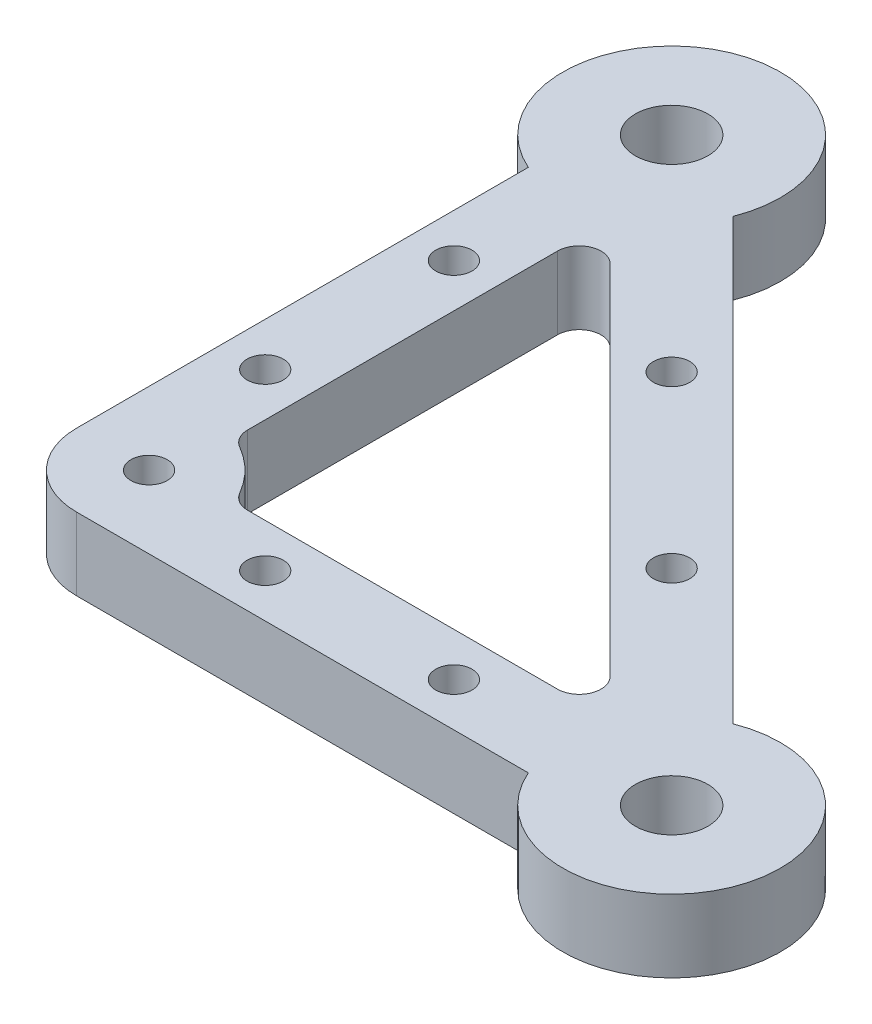
ISO-10303-21;
HEADER;
FILE_DESCRIPTION(('STEP AP214'),'2;1');
FILE_NAME('part.step','',(''),(''),'','','');
FILE_SCHEMA(('AUTOMOTIVE_DESIGN { 1 0 10303 214 1 1 1 1 }'));
ENDSEC;
DATA;
#1=APPLICATION_CONTEXT('core data for automotive mechanical design processes');
#2=APPLICATION_PROTOCOL_DEFINITION('international standard','automotive_design',2000,#1);
#3=PRODUCT_CONTEXT('',#1,'mechanical');
#4=PRODUCT('Part','Part','',(#3));
#5=PRODUCT_RELATED_PRODUCT_CATEGORY('part','',(#4));
#6=PRODUCT_DEFINITION_FORMATION('','',#4);
#7=PRODUCT_DEFINITION_CONTEXT('part definition',#1,'design');
#8=PRODUCT_DEFINITION('design','',#6,#7);
#9=PRODUCT_DEFINITION_SHAPE('','',#8);
#10=(LENGTH_UNIT() NAMED_UNIT(*) SI_UNIT(.MILLI.,.METRE.));
#11=(NAMED_UNIT(*) PLANE_ANGLE_UNIT() SI_UNIT($,.RADIAN.));
#12=(NAMED_UNIT(*) SI_UNIT($,.STERADIAN.) SOLID_ANGLE_UNIT());
#13=UNCERTAINTY_MEASURE_WITH_UNIT(LENGTH_MEASURE(1.E-05),#10,'distance_accuracy_value','');
#14=(GEOMETRIC_REPRESENTATION_CONTEXT(3) GLOBAL_UNCERTAINTY_ASSIGNED_CONTEXT((#13)) GLOBAL_UNIT_ASSIGNED_CONTEXT((#10,
#11,#12)) REPRESENTATION_CONTEXT('',''));
#15=CARTESIAN_POINT('',(0.,0.,0.));
#16=DIRECTION('',(0.,0.,1.));
#17=DIRECTION('',(1.,0.,0.));
#18=AXIS2_PLACEMENT_3D('',#15,#16,#17);
#19=CARTESIAN_POINT('',(4.,5.,-4.));
#20=DIRECTION('',(0.,1.,0.));
#21=DIRECTION('',(0.,0.,1.));
#22=AXIS2_PLACEMENT_3D('',#19,#20,#21);
#23=PLANE('',#22);
#24=CARTESIAN_POINT('',(28.2842712474619,5.,-51.7157287525381));
#25=DIRECTION('',(0.,1.,0.));
#26=DIRECTION('',(0.,0.,1.));
#27=AXIS2_PLACEMENT_3D('',#24,#25,#26);
#28=CIRCLE('',#27,2.5);
#29=CARTESIAN_POINT('',(28.2842712474619,5.,-49.2157287525381));
#30=VERTEX_POINT('',#29);
#31=EDGE_CURVE('E389',#30,#30,#28,.T.);
#32=ORIENTED_EDGE('',*,*,#31,.F.);
#33=EDGE_LOOP('',(#32));
#34=FACE_BOUND('',#33,.T.);
#35=CARTESIAN_POINT('',(0.,5.,-24.));
#36=DIRECTION('',(0.,1.,0.));
#37=DIRECTION('',(0.,0.,1.));
#38=AXIS2_PLACEMENT_3D('',#35,#36,#37);
#39=CIRCLE('',#38,2.5);
#40=CARTESIAN_POINT('',(0.,5.,-21.5));
#41=VERTEX_POINT('',#40);
#42=EDGE_CURVE('E398',#41,#41,#39,.T.);
#43=ORIENTED_EDGE('',*,*,#42,.F.);
#44=EDGE_LOOP('',(#43));
#45=FACE_BOUND('',#44,.T.);
#46=CARTESIAN_POINT('',(50.,5.,0.));
#47=DIRECTION('',(0.,1.,0.));
#48=DIRECTION('',(0.,0.,1.));
#49=AXIS2_PLACEMENT_3D('',#46,#47,#48);
#50=CIRCLE('',#49,2.5);
#51=CARTESIAN_POINT('',(50.,5.,2.5));
#52=VERTEX_POINT('',#51);
#53=EDGE_CURVE('E179',#52,#52,#50,.T.);
#54=ORIENTED_EDGE('',*,*,#53,.F.);
#55=EDGE_LOOP('',(#54));
#56=FACE_BOUND('',#55,.T.);
#57=CARTESIAN_POINT('',(0.,5.,-80.));
#58=DIRECTION('',(0.,1.,0.));
#59=DIRECTION('',(0.,0.,1.));
#60=AXIS2_PLACEMENT_3D('',#57,#58,#59);
#61=CIRCLE('',#60,5.);
#62=CARTESIAN_POINT('',(0.,5.,-75.));
#63=VERTEX_POINT('',#62);
#64=EDGE_CURVE('E212',#63,#63,#61,.T.);
#65=ORIENTED_EDGE('',*,*,#64,.F.);
#66=EDGE_LOOP('',(#65));
#67=FACE_BOUND('',#66,.T.);
#68=CARTESIAN_POINT('',(4.,5.,-4.));
#69=DIRECTION('',(0.,1.,0.));
#70=DIRECTION('',(0.,0.,1.));
#71=AXIS2_PLACEMENT_3D('',#68,#69,#70);
#72=CIRCLE('',#71,10.);
#73=CARTESIAN_POINT('',(-6.,5.,-4.));
#74=VERTEX_POINT('',#73);
#75=CARTESIAN_POINT('',(4.,5.,6.));
#76=VERTEX_POINT('',#75);
#77=EDGE_CURVE('E227',#74,#76,#72,.T.);
#78=ORIENTED_EDGE('',*,*,#77,.T.);
#79=DIRECTION('',(1.,0.,0.));
#80=VECTOR('',#79,1.);
#81=CARTESIAN_POINT('',(4.,5.,6.));
#82=LINE('',#81,#80);
#83=CARTESIAN_POINT('',(66.2522729151325,5.,5.99999999999999));
#84=VERTEX_POINT('',#83);
#85=EDGE_CURVE('E226',#76,#84,#82,.T.);
#86=ORIENTED_EDGE('',*,*,#85,.T.);
#87=CARTESIAN_POINT('',(80.,5.,0.));
#88=DIRECTION('',(0.,1.,0.));
#89=DIRECTION('',(0.,0.,1.));
#90=AXIS2_PLACEMENT_3D('',#87,#88,#89);
#91=CIRCLE('',#90,15.);
#92=CARTESIAN_POINT('',(74.5215296395075,5.,-13.9637517347311));
#93=VERTEX_POINT('',#92);
#94=EDGE_CURVE('E235',#84,#93,#91,.T.);
#95=ORIENTED_EDGE('',*,*,#94,.T.);
#96=DIRECTION('',(-0.707106781186547,0.,-0.707106781186547));
#97=VECTOR('',#96,1.);
#98=CARTESIAN_POINT('',(13.9637517347311,5.,-74.5215296395075));
#99=LINE('',#98,#97);
#100=CARTESIAN_POINT('',(13.9637517347311,5.,-74.5215296395075));
#101=VERTEX_POINT('',#100);
#102=EDGE_CURVE('E231',#93,#101,#99,.T.);
#103=ORIENTED_EDGE('',*,*,#102,.T.);
#104=CARTESIAN_POINT('',(0.,5.,-80.));
#105=DIRECTION('',(0.,1.,0.));
#106=DIRECTION('',(0.,0.,1.));
#107=AXIS2_PLACEMENT_3D('',#104,#105,#106);
#108=CIRCLE('',#107,15.);
#109=CARTESIAN_POINT('',(-6.,5.,-66.2522729151325));
#110=VERTEX_POINT('',#109);
#111=EDGE_CURVE('E237',#101,#110,#108,.T.);
#112=ORIENTED_EDGE('',*,*,#111,.T.);
#113=DIRECTION('',(0.,0.,1.));
#114=VECTOR('',#113,1.);
#115=CARTESIAN_POINT('',(-6.,5.,-4.));
#116=LINE('',#115,#114);
#117=EDGE_CURVE('E236',#110,#74,#116,.T.);
#118=ORIENTED_EDGE('',*,*,#117,.T.);
#119=EDGE_LOOP('',(#78,#86,#95,#103,#112,#118));
#120=FACE_BOUND('',#119,.T.);
#121=CARTESIAN_POINT('',(80.,5.,0.));
#122=DIRECTION('',(0.,1.,0.));
#123=DIRECTION('',(0.,0.,1.));
#124=AXIS2_PLACEMENT_3D('',#121,#122,#123);
#125=CIRCLE('',#124,5.);
#126=CARTESIAN_POINT('',(80.,5.,5.));
#127=VERTEX_POINT('',#126);
#128=EDGE_CURVE('E219',#127,#127,#125,.T.);
#129=ORIENTED_EDGE('',*,*,#128,.F.);
#130=EDGE_LOOP('',(#129));
#131=FACE_BOUND('',#130,.T.);
#132=CARTESIAN_POINT('',(4.,5.,-4.));
#133=DIRECTION('',(0.,1.,0.));
#134=DIRECTION('',(0.,0.,1.));
#135=AXIS2_PLACEMENT_3D('',#132,#133,#134);
#136=CIRCLE('',#135,2.5);
#137=CARTESIAN_POINT('',(4.,5.,-1.5));
#138=VERTEX_POINT('',#137);
#139=EDGE_CURVE('E208',#138,#138,#136,.T.);
#140=ORIENTED_EDGE('',*,*,#139,.F.);
#141=EDGE_LOOP('',(#140));
#142=FACE_BOUND('',#141,.T.);
#143=DIRECTION('',(1.,0.,0.));
#144=VECTOR('',#143,1.);
#145=CARTESIAN_POINT('',(15.5884572681199,5.,-6.));
#146=LINE('',#145,#144);
#147=CARTESIAN_POINT('',(15.5884572681199,5.,-6.));
#148=VERTEX_POINT('',#147);
#149=CARTESIAN_POINT('',(58.2720779386422,5.,-6.));
#150=VERTEX_POINT('',#149);
#151=EDGE_CURVE('E146',#148,#150,#146,.T.);
#152=ORIENTED_EDGE('',*,*,#151,.F.);
#153=CARTESIAN_POINT('',(15.5884572681199,5.,-9.));
#154=DIRECTION('',(0.,1.,0.));
#155=DIRECTION('',(0.,0.,-1.));
#156=AXIS2_PLACEMENT_3D('',#153,#154,#155);
#157=CIRCLE('',#156,3.);
#158=CARTESIAN_POINT('',(12.9903810567666,5.,-7.5));
#159=VERTEX_POINT('',#158);
#160=EDGE_CURVE('E138',#159,#148,#157,.T.);
#161=ORIENTED_EDGE('',*,*,#160,.F.);
#162=CARTESIAN_POINT('',(0.,5.,0.));
#163=DIRECTION('',(0.,-1.,0.));
#164=DIRECTION('',(0.,0.,1.));
#165=AXIS2_PLACEMENT_3D('',#162,#163,#164);
#166=CIRCLE('',#165,15.);
#167=CARTESIAN_POINT('',(7.5,5.,-12.9903810567666));
#168=VERTEX_POINT('',#167);
#169=EDGE_CURVE('E173',#168,#159,#166,.T.);
#170=ORIENTED_EDGE('',*,*,#169,.F.);
#171=CARTESIAN_POINT('',(9.,5.,-15.5884572681199));
#172=DIRECTION('',(0.,1.,0.));
#173=DIRECTION('',(0.,0.,-1.));
#174=AXIS2_PLACEMENT_3D('',#171,#172,#173);
#175=CIRCLE('',#174,3.);
#176=CARTESIAN_POINT('',(6.,5.,-15.5884572681199));
#177=VERTEX_POINT('',#176);
#178=EDGE_CURVE('E174',#177,#168,#175,.T.);
#179=ORIENTED_EDGE('',*,*,#178,.F.);
#180=DIRECTION('',(0.,0.,1.));
#181=VECTOR('',#180,1.);
#182=CARTESIAN_POINT('',(6.,5.,-15.5884572681199));
#183=LINE('',#182,#181);
#184=CARTESIAN_POINT('',(6.,5.,-58.2720779386421));
#185=VERTEX_POINT('',#184);
#186=EDGE_CURVE('E172',#185,#177,#183,.T.);
#187=ORIENTED_EDGE('',*,*,#186,.F.);
#188=CARTESIAN_POINT('',(9.,5.,-58.2720779386421));
#189=DIRECTION('',(0.,1.,0.));
#190=DIRECTION('',(0.,0.,1.));
#191=AXIS2_PLACEMENT_3D('',#188,#189,#190);
#192=CIRCLE('',#191,3.);
#193=CARTESIAN_POINT('',(11.1213203435596,5.,-60.3933982822018));
#194=VERTEX_POINT('',#193);
#195=EDGE_CURVE('E166',#194,#185,#192,.T.);
#196=ORIENTED_EDGE('',*,*,#195,.F.);
#197=DIRECTION('',(-0.707106781186547,0.,-0.707106781186547));
#198=VECTOR('',#197,1.);
#199=CARTESIAN_POINT('',(11.1213203435596,5.,-60.3933982822018));
#200=LINE('',#199,#198);
#201=CARTESIAN_POINT('',(60.3933982822018,5.,-11.1213203435596));
#202=VERTEX_POINT('',#201);
#203=EDGE_CURVE('E163',#202,#194,#200,.T.);
#204=ORIENTED_EDGE('',*,*,#203,.F.);
#205=CARTESIAN_POINT('',(58.2720779386422,5.,-9.));
#206=DIRECTION('',(0.,1.,0.));
#207=DIRECTION('',(0.,0.,1.));
#208=AXIS2_PLACEMENT_3D('',#205,#206,#207);
#209=CIRCLE('',#208,3.);
#210=EDGE_CURVE('E165',#150,#202,#209,.T.);
#211=ORIENTED_EDGE('',*,*,#210,.F.);
#212=EDGE_LOOP('',(#152,#161,#170,#179,#187,#196,#204,#211));
#213=FACE_BOUND('',#212,.T.);
#214=CARTESIAN_POINT('',(24.,5.,0.));
#215=DIRECTION('',(0.,1.,0.));
#216=DIRECTION('',(0.,0.,1.));
#217=AXIS2_PLACEMENT_3D('',#214,#215,#216);
#218=CIRCLE('',#217,2.5);
#219=CARTESIAN_POINT('',(24.,5.,2.5));
#220=VERTEX_POINT('',#219);
#221=EDGE_CURVE('E407',#220,#220,#218,.T.);
#222=ORIENTED_EDGE('',*,*,#221,.F.);
#223=EDGE_LOOP('',(#222));
#224=FACE_BOUND('',#223,.T.);
#225=CARTESIAN_POINT('',(0.,5.,-50.));
#226=DIRECTION('',(0.,1.,0.));
#227=DIRECTION('',(0.,0.,1.));
#228=AXIS2_PLACEMENT_3D('',#225,#226,#227);
#229=CIRCLE('',#228,2.5);
#230=CARTESIAN_POINT('',(0.,5.,-47.5));
#231=VERTEX_POINT('',#230);
#232=EDGE_CURVE('E391',#231,#231,#229,.T.);
#233=ORIENTED_EDGE('',*,*,#232,.F.);
#234=EDGE_LOOP('',(#233));
#235=FACE_BOUND('',#234,.T.);
#236=CARTESIAN_POINT('',(51.7157287525381,5.,-28.2842712474619));
#237=DIRECTION('',(0.,1.,0.));
#238=DIRECTION('',(0.,0.,1.));
#239=AXIS2_PLACEMENT_3D('',#236,#237,#238);
#240=CIRCLE('',#239,2.5);
#241=CARTESIAN_POINT('',(51.7157287525381,5.,-25.7842712474619));
#242=VERTEX_POINT('',#241);
#243=EDGE_CURVE('E377',#242,#242,#240,.T.);
#244=ORIENTED_EDGE('',*,*,#243,.F.);
#245=EDGE_LOOP('',(#244));
#246=FACE_BOUND('',#245,.T.);
#247=ADVANCED_FACE('F39',(#34,#45,#56,#67,#120,#131,#142,#213,#224,#235,#246),#23,.T.);
#248=CARTESIAN_POINT('',(4.,-5.,-4.));
#249=DIRECTION('',(0.,1.,0.));
#250=DIRECTION('',(0.,0.,1.));
#251=AXIS2_PLACEMENT_3D('',#248,#249,#250);
#252=PLANE('',#251);
#253=CARTESIAN_POINT('',(4.,-5.,-4.));
#254=DIRECTION('',(0.,1.,0.));
#255=DIRECTION('',(0.,0.,1.));
#256=AXIS2_PLACEMENT_3D('',#253,#254,#255);
#257=CIRCLE('',#256,2.5);
#258=CARTESIAN_POINT('',(4.,-5.,-1.5));
#259=VERTEX_POINT('',#258);
#260=EDGE_CURVE('E156',#259,#259,#257,.T.);
#261=ORIENTED_EDGE('',*,*,#260,.T.);
#262=EDGE_LOOP('',(#261));
#263=FACE_BOUND('',#262,.T.);
#264=CARTESIAN_POINT('',(0.,-5.,-80.));
#265=DIRECTION('',(0.,1.,0.));
#266=DIRECTION('',(0.,0.,1.));
#267=AXIS2_PLACEMENT_3D('',#264,#265,#266);
#268=CIRCLE('',#267,5.);
#269=CARTESIAN_POINT('',(0.,-5.,-75.));
#270=VERTEX_POINT('',#269);
#271=EDGE_CURVE('E211',#270,#270,#268,.T.);
#272=ORIENTED_EDGE('',*,*,#271,.T.);
#273=EDGE_LOOP('',(#272));
#274=FACE_BOUND('',#273,.T.);
#275=CARTESIAN_POINT('',(80.,-5.,0.));
#276=DIRECTION('',(0.,1.,0.));
#277=DIRECTION('',(0.,0.,1.));
#278=AXIS2_PLACEMENT_3D('',#275,#276,#277);
#279=CIRCLE('',#278,5.);
#280=CARTESIAN_POINT('',(80.,-5.,5.));
#281=VERTEX_POINT('',#280);
#282=EDGE_CURVE('E220',#281,#281,#279,.T.);
#283=ORIENTED_EDGE('',*,*,#282,.T.);
#284=EDGE_LOOP('',(#283));
#285=FACE_BOUND('',#284,.T.);
#286=CARTESIAN_POINT('',(4.,-5.,-4.));
#287=DIRECTION('',(0.,1.,0.));
#288=DIRECTION('',(0.,0.,1.));
#289=AXIS2_PLACEMENT_3D('',#286,#287,#288);
#290=CIRCLE('',#289,10.);
#291=CARTESIAN_POINT('',(-6.,-5.,-4.));
#292=VERTEX_POINT('',#291);
#293=CARTESIAN_POINT('',(4.,-5.,6.));
#294=VERTEX_POINT('',#293);
#295=EDGE_CURVE('E224',#292,#294,#290,.T.);
#296=ORIENTED_EDGE('',*,*,#295,.F.);
#297=DIRECTION('',(0.,0.,1.));
#298=VECTOR('',#297,1.);
#299=CARTESIAN_POINT('',(-6.,-5.,-4.));
#300=LINE('',#299,#298);
#301=CARTESIAN_POINT('',(-6.,-5.,-66.2522729151325));
#302=VERTEX_POINT('',#301);
#303=EDGE_CURVE('E228',#302,#292,#300,.T.);
#304=ORIENTED_EDGE('',*,*,#303,.F.);
#305=CARTESIAN_POINT('',(0.,-5.,-80.));
#306=DIRECTION('',(0.,1.,0.));
#307=DIRECTION('',(0.,0.,1.));
#308=AXIS2_PLACEMENT_3D('',#305,#306,#307);
#309=CIRCLE('',#308,15.);
#310=CARTESIAN_POINT('',(13.9637517347311,-5.,-74.5215296395075));
#311=VERTEX_POINT('',#310);
#312=EDGE_CURVE('E246',#311,#302,#309,.T.);
#313=ORIENTED_EDGE('',*,*,#312,.F.);
#314=DIRECTION('',(-0.707106781186547,0.,-0.707106781186547));
#315=VECTOR('',#314,1.);
#316=CARTESIAN_POINT('',(13.9637517347311,-5.,-74.5215296395075));
#317=LINE('',#316,#315);
#318=CARTESIAN_POINT('',(74.5215296395075,-5.,-13.9637517347311));
#319=VERTEX_POINT('',#318);
#320=EDGE_CURVE('E250',#319,#311,#317,.T.);
#321=ORIENTED_EDGE('',*,*,#320,.F.);
#322=CARTESIAN_POINT('',(80.,-5.,0.));
#323=DIRECTION('',(0.,1.,0.));
#324=DIRECTION('',(0.,0.,1.));
#325=AXIS2_PLACEMENT_3D('',#322,#323,#324);
#326=CIRCLE('',#325,15.);
#327=CARTESIAN_POINT('',(66.2522729151325,-5.,5.99999999999999));
#328=VERTEX_POINT('',#327);
#329=EDGE_CURVE('E243',#328,#319,#326,.T.);
#330=ORIENTED_EDGE('',*,*,#329,.F.);
#331=DIRECTION('',(1.,0.,0.));
#332=VECTOR('',#331,1.);
#333=CARTESIAN_POINT('',(4.,-5.,6.));
#334=LINE('',#333,#332);
#335=EDGE_CURVE('E244',#294,#328,#334,.T.);
#336=ORIENTED_EDGE('',*,*,#335,.F.);
#337=EDGE_LOOP('',(#296,#304,#313,#321,#330,#336));
#338=FACE_BOUND('',#337,.T.);
#339=CARTESIAN_POINT('',(15.5884572681199,-5.,-9.));
#340=DIRECTION('',(0.,1.,0.));
#341=DIRECTION('',(0.,0.,-1.));
#342=AXIS2_PLACEMENT_3D('',#339,#340,#341);
#343=CIRCLE('',#342,3.);
#344=CARTESIAN_POINT('',(12.9903810567666,-5.,-7.5));
#345=VERTEX_POINT('',#344);
#346=CARTESIAN_POINT('',(15.5884572681199,-5.,-6.));
#347=VERTEX_POINT('',#346);
#348=EDGE_CURVE('E65',#345,#347,#343,.T.);
#349=ORIENTED_EDGE('',*,*,#348,.T.);
#350=DIRECTION('',(1.,0.,0.));
#351=VECTOR('',#350,1.);
#352=CARTESIAN_POINT('',(15.5884572681199,-5.,-6.));
#353=LINE('',#352,#351);
#354=CARTESIAN_POINT('',(58.2720779386422,-5.,-6.));
#355=VERTEX_POINT('',#354);
#356=EDGE_CURVE('E154',#347,#355,#353,.T.);
#357=ORIENTED_EDGE('',*,*,#356,.T.);
#358=CARTESIAN_POINT('',(58.2720779386422,-5.,-9.));
#359=DIRECTION('',(0.,1.,0.));
#360=DIRECTION('',(0.,0.,1.));
#361=AXIS2_PLACEMENT_3D('',#358,#359,#360);
#362=CIRCLE('',#361,3.);
#363=CARTESIAN_POINT('',(60.3933982822018,-5.,-11.1213203435596));
#364=VERTEX_POINT('',#363);
#365=EDGE_CURVE('E178',#355,#364,#362,.T.);
#366=ORIENTED_EDGE('',*,*,#365,.T.);
#367=DIRECTION('',(-0.707106781186547,0.,-0.707106781186547));
#368=VECTOR('',#367,1.);
#369=CARTESIAN_POINT('',(11.1213203435596,-5.,-60.3933982822018));
#370=LINE('',#369,#368);
#371=CARTESIAN_POINT('',(11.1213203435596,-5.,-60.3933982822018));
#372=VERTEX_POINT('',#371);
#373=EDGE_CURVE('E181',#364,#372,#370,.T.);
#374=ORIENTED_EDGE('',*,*,#373,.T.);
#375=CARTESIAN_POINT('',(9.,-5.,-58.2720779386421));
#376=DIRECTION('',(0.,1.,0.));
#377=DIRECTION('',(0.,0.,1.));
#378=AXIS2_PLACEMENT_3D('',#375,#376,#377);
#379=CIRCLE('',#378,3.);
#380=CARTESIAN_POINT('',(6.,-5.,-58.2720779386421));
#381=VERTEX_POINT('',#380);
#382=EDGE_CURVE('E187',#372,#381,#379,.T.);
#383=ORIENTED_EDGE('',*,*,#382,.T.);
#384=DIRECTION('',(0.,0.,1.));
#385=VECTOR('',#384,1.);
#386=CARTESIAN_POINT('',(6.,-5.,-15.5884572681199));
#387=LINE('',#386,#385);
#388=CARTESIAN_POINT('',(6.,-5.,-15.5884572681199));
#389=VERTEX_POINT('',#388);
#390=EDGE_CURVE('E186',#381,#389,#387,.T.);
#391=ORIENTED_EDGE('',*,*,#390,.T.);
#392=CARTESIAN_POINT('',(9.,-5.,-15.5884572681199));
#393=DIRECTION('',(0.,1.,0.));
#394=DIRECTION('',(0.,0.,-1.));
#395=AXIS2_PLACEMENT_3D('',#392,#393,#394);
#396=CIRCLE('',#395,3.);
#397=CARTESIAN_POINT('',(7.5,-5.,-12.9903810567666));
#398=VERTEX_POINT('',#397);
#399=EDGE_CURVE('E195',#389,#398,#396,.T.);
#400=ORIENTED_EDGE('',*,*,#399,.T.);
#401=CARTESIAN_POINT('',(0.,-5.,0.));
#402=DIRECTION('',(0.,-1.,0.));
#403=DIRECTION('',(0.,0.,1.));
#404=AXIS2_PLACEMENT_3D('',#401,#402,#403);
#405=CIRCLE('',#404,15.);
#406=EDGE_CURVE('E149',#398,#345,#405,.T.);
#407=ORIENTED_EDGE('',*,*,#406,.T.);
#408=EDGE_LOOP('',(#349,#357,#366,#374,#383,#391,#400,#407));
#409=FACE_BOUND('',#408,.T.);
#410=CARTESIAN_POINT('',(50.,-5.,0.));
#411=DIRECTION('',(0.,1.,0.));
#412=DIRECTION('',(0.,0.,1.));
#413=AXIS2_PLACEMENT_3D('',#410,#411,#412);
#414=CIRCLE('',#413,2.5);
#415=CARTESIAN_POINT('',(50.,-5.,2.5));
#416=VERTEX_POINT('',#415);
#417=EDGE_CURVE('E406',#416,#416,#414,.T.);
#418=ORIENTED_EDGE('',*,*,#417,.T.);
#419=EDGE_LOOP('',(#418));
#420=FACE_BOUND('',#419,.T.);
#421=CARTESIAN_POINT('',(24.,-5.,0.));
#422=DIRECTION('',(0.,1.,0.));
#423=DIRECTION('',(0.,0.,1.));
#424=AXIS2_PLACEMENT_3D('',#421,#422,#423);
#425=CIRCLE('',#424,2.5);
#426=CARTESIAN_POINT('',(24.,-5.,2.5));
#427=VERTEX_POINT('',#426);
#428=EDGE_CURVE('E401',#427,#427,#425,.T.);
#429=ORIENTED_EDGE('',*,*,#428,.T.);
#430=EDGE_LOOP('',(#429));
#431=FACE_BOUND('',#430,.T.);
#432=CARTESIAN_POINT('',(0.,-5.,-24.));
#433=DIRECTION('',(0.,1.,0.));
#434=DIRECTION('',(0.,0.,1.));
#435=AXIS2_PLACEMENT_3D('',#432,#433,#434);
#436=CIRCLE('',#435,2.5);
#437=CARTESIAN_POINT('',(0.,-5.,-21.5));
#438=VERTEX_POINT('',#437);
#439=EDGE_CURVE('E400',#438,#438,#436,.T.);
#440=ORIENTED_EDGE('',*,*,#439,.T.);
#441=EDGE_LOOP('',(#440));
#442=FACE_BOUND('',#441,.T.);
#443=CARTESIAN_POINT('',(0.,-5.,-50.));
#444=DIRECTION('',(0.,1.,0.));
#445=DIRECTION('',(0.,0.,1.));
#446=AXIS2_PLACEMENT_3D('',#443,#444,#445);
#447=CIRCLE('',#446,2.5);
#448=CARTESIAN_POINT('',(0.,-5.,-47.5));
#449=VERTEX_POINT('',#448);
#450=EDGE_CURVE('E392',#449,#449,#447,.T.);
#451=ORIENTED_EDGE('',*,*,#450,.T.);
#452=EDGE_LOOP('',(#451));
#453=FACE_BOUND('',#452,.T.);
#454=CARTESIAN_POINT('',(28.2842712474619,-5.,-51.7157287525381));
#455=DIRECTION('',(0.,1.,0.));
#456=DIRECTION('',(0.,0.,1.));
#457=AXIS2_PLACEMENT_3D('',#454,#455,#456);
#458=CIRCLE('',#457,2.5);
#459=CARTESIAN_POINT('',(28.2842712474619,-5.,-49.2157287525381));
#460=VERTEX_POINT('',#459);
#461=EDGE_CURVE('E384',#460,#460,#458,.T.);
#462=ORIENTED_EDGE('',*,*,#461,.T.);
#463=EDGE_LOOP('',(#462));
#464=FACE_BOUND('',#463,.T.);
#465=CARTESIAN_POINT('',(51.7157287525381,-5.,-28.2842712474619));
#466=DIRECTION('',(0.,1.,0.));
#467=DIRECTION('',(0.,0.,1.));
#468=AXIS2_PLACEMENT_3D('',#465,#466,#467);
#469=CIRCLE('',#468,2.5);
#470=CARTESIAN_POINT('',(51.7157287525381,-5.,-25.7842712474619));
#471=VERTEX_POINT('',#470);
#472=EDGE_CURVE('E385',#471,#471,#469,.T.);
#473=ORIENTED_EDGE('',*,*,#472,.T.);
#474=EDGE_LOOP('',(#473));
#475=FACE_BOUND('',#474,.T.);
#476=ADVANCED_FACE('F272',(#263,#274,#285,#338,#409,#420,#431,#442,#453,#464,#475),#252,.F.);
#477=CARTESIAN_POINT('',(4.,5.,-4.));
#478=DIRECTION('',(0.,-1.,0.));
#479=DIRECTION('',(0.,0.,-1.));
#480=AXIS2_PLACEMENT_3D('',#477,#478,#479);
#481=CYLINDRICAL_SURFACE('',#480,10.);
#482=ORIENTED_EDGE('',*,*,#295,.T.);
#483=DIRECTION('',(0.,-1.,0.));
#484=VECTOR('',#483,1.);
#485=CARTESIAN_POINT('',(4.,5.,6.));
#486=LINE('',#485,#484);
#487=EDGE_CURVE('E11',#76,#294,#486,.T.);
#488=ORIENTED_EDGE('',*,*,#487,.F.);
#489=ORIENTED_EDGE('',*,*,#77,.F.);
#490=DIRECTION('',(0.,-1.,0.));
#491=VECTOR('',#490,1.);
#492=CARTESIAN_POINT('',(-6.,5.,-4.));
#493=LINE('',#492,#491);
#494=EDGE_CURVE('E238',#74,#292,#493,.T.);
#495=ORIENTED_EDGE('',*,*,#494,.T.);
#496=EDGE_LOOP('',(#482,#488,#489,#495));
#497=FACE_BOUND('',#496,.T.);
#498=ADVANCED_FACE('F41',(#497),#481,.T.);
#499=CARTESIAN_POINT('',(4.,5.,6.));
#500=DIRECTION('',(0.,0.,-1.));
#501=DIRECTION('',(-1.,0.,0.));
#502=AXIS2_PLACEMENT_3D('',#499,#500,#501);
#503=PLANE('',#502);
#504=ORIENTED_EDGE('',*,*,#335,.T.);
#505=DIRECTION('',(0.,-1.,0.));
#506=VECTOR('',#505,1.);
#507=CARTESIAN_POINT('',(66.2522729151325,5.,5.99999999999999));
#508=LINE('',#507,#506);
#509=EDGE_CURVE('E50',#84,#328,#508,.T.);
#510=ORIENTED_EDGE('',*,*,#509,.F.);
#511=ORIENTED_EDGE('',*,*,#85,.F.);
#512=ORIENTED_EDGE('',*,*,#487,.T.);
#513=EDGE_LOOP('',(#504,#510,#511,#512));
#514=FACE_BOUND('',#513,.T.);
#515=ADVANCED_FACE('F292',(#514),#503,.F.);
#516=CARTESIAN_POINT('',(80.,5.,0.));
#517=DIRECTION('',(0.,-1.,0.));
#518=DIRECTION('',(0.,0.,-1.));
#519=AXIS2_PLACEMENT_3D('',#516,#517,#518);
#520=CYLINDRICAL_SURFACE('',#519,15.);
#521=ORIENTED_EDGE('',*,*,#329,.T.);
#522=DIRECTION('',(0.,-1.,0.));
#523=VECTOR('',#522,1.);
#524=CARTESIAN_POINT('',(74.5215296395075,5.,-13.9637517347311));
#525=LINE('',#524,#523);
#526=EDGE_CURVE('E257',#93,#319,#525,.T.);
#527=ORIENTED_EDGE('',*,*,#526,.F.);
#528=ORIENTED_EDGE('',*,*,#94,.F.);
#529=ORIENTED_EDGE('',*,*,#509,.T.);
#530=EDGE_LOOP('',(#521,#527,#528,#529));
#531=FACE_BOUND('',#530,.T.);
#532=ADVANCED_FACE('F270',(#531),#520,.T.);
#533=CARTESIAN_POINT('',(13.9637517347311,5.,-74.5215296395075));
#534=DIRECTION('',(-0.707106781186548,0.,0.707106781186548));
#535=DIRECTION('',(0.707106781186548,0.,0.707106781186548));
#536=AXIS2_PLACEMENT_3D('',#533,#534,#535);
#537=PLANE('',#536);
#538=ORIENTED_EDGE('',*,*,#320,.T.);
#539=DIRECTION('',(0.,-1.,0.));
#540=VECTOR('',#539,1.);
#541=CARTESIAN_POINT('',(13.9637517347311,5.,-74.5215296395075));
#542=LINE('',#541,#540);
#543=EDGE_CURVE('E260',#101,#311,#542,.T.);
#544=ORIENTED_EDGE('',*,*,#543,.F.);
#545=ORIENTED_EDGE('',*,*,#102,.F.);
#546=ORIENTED_EDGE('',*,*,#526,.T.);
#547=EDGE_LOOP('',(#538,#544,#545,#546));
#548=FACE_BOUND('',#547,.T.);
#549=ADVANCED_FACE('F276',(#548),#537,.F.);
#550=CARTESIAN_POINT('',(0.,5.,-80.));
#551=DIRECTION('',(0.,-1.,0.));
#552=DIRECTION('',(0.,0.,-1.));
#553=AXIS2_PLACEMENT_3D('',#550,#551,#552);
#554=CYLINDRICAL_SURFACE('',#553,15.);
#555=ORIENTED_EDGE('',*,*,#312,.T.);
#556=DIRECTION('',(0.,-1.,0.));
#557=VECTOR('',#556,1.);
#558=CARTESIAN_POINT('',(-6.,5.,-66.2522729151325));
#559=LINE('',#558,#557);
#560=EDGE_CURVE('E255',#110,#302,#559,.T.);
#561=ORIENTED_EDGE('',*,*,#560,.F.);
#562=ORIENTED_EDGE('',*,*,#111,.F.);
#563=ORIENTED_EDGE('',*,*,#543,.T.);
#564=EDGE_LOOP('',(#555,#561,#562,#563));
#565=FACE_BOUND('',#564,.T.);
#566=ADVANCED_FACE('F284',(#565),#554,.T.);
#567=CARTESIAN_POINT('',(-6.,5.,-4.));
#568=DIRECTION('',(1.,0.,0.));
#569=DIRECTION('',(0.,0.,-1.));
#570=AXIS2_PLACEMENT_3D('',#567,#568,#569);
#571=PLANE('',#570);
#572=ORIENTED_EDGE('',*,*,#303,.T.);
#573=ORIENTED_EDGE('',*,*,#494,.F.);
#574=ORIENTED_EDGE('',*,*,#117,.F.);
#575=ORIENTED_EDGE('',*,*,#560,.T.);
#576=EDGE_LOOP('',(#572,#573,#574,#575));
#577=FACE_BOUND('',#576,.T.);
#578=ADVANCED_FACE('F294',(#577),#571,.F.);
#579=CARTESIAN_POINT('',(80.,5.,0.));
#580=DIRECTION('',(0.,-1.,0.));
#581=DIRECTION('',(0.,0.,-1.));
#582=AXIS2_PLACEMENT_3D('',#579,#580,#581);
#583=CYLINDRICAL_SURFACE('',#582,5.);
#584=ORIENTED_EDGE('',*,*,#128,.T.);
#585=EDGE_LOOP('',(#584));
#586=FACE_BOUND('',#585,.T.);
#587=ORIENTED_EDGE('',*,*,#282,.F.);
#588=EDGE_LOOP('',(#587));
#589=FACE_BOUND('',#588,.T.);
#590=ADVANCED_FACE('F297',(#586,#589),#583,.F.);
#591=CARTESIAN_POINT('',(0.,5.,-80.));
#592=DIRECTION('',(0.,-1.,0.));
#593=DIRECTION('',(0.,0.,-1.));
#594=AXIS2_PLACEMENT_3D('',#591,#592,#593);
#595=CYLINDRICAL_SURFACE('',#594,5.);
#596=ORIENTED_EDGE('',*,*,#64,.T.);
#597=EDGE_LOOP('',(#596));
#598=FACE_BOUND('',#597,.T.);
#599=ORIENTED_EDGE('',*,*,#271,.F.);
#600=EDGE_LOOP('',(#599));
#601=FACE_BOUND('',#600,.T.);
#602=ADVANCED_FACE('F305',(#598,#601),#595,.F.);
#603=CARTESIAN_POINT('',(4.,5.,-4.));
#604=DIRECTION('',(0.,-1.,0.));
#605=DIRECTION('',(0.,0.,-1.));
#606=AXIS2_PLACEMENT_3D('',#603,#604,#605);
#607=CYLINDRICAL_SURFACE('',#606,2.5);
#608=ORIENTED_EDGE('',*,*,#139,.T.);
#609=EDGE_LOOP('',(#608));
#610=FACE_BOUND('',#609,.T.);
#611=ORIENTED_EDGE('',*,*,#260,.F.);
#612=EDGE_LOOP('',(#611));
#613=FACE_BOUND('',#612,.T.);
#614=ADVANCED_FACE('F317',(#610,#613),#607,.F.);
#615=CARTESIAN_POINT('',(15.5884572681199,5.,-9.));
#616=DIRECTION('',(0.,-1.,0.));
#617=DIRECTION('',(0.,0.,-1.));
#618=AXIS2_PLACEMENT_3D('',#615,#616,#617);
#619=CYLINDRICAL_SURFACE('',#618,3.);
#620=ORIENTED_EDGE('',*,*,#348,.F.);
#621=DIRECTION('',(0.,-1.,0.));
#622=VECTOR('',#621,1.);
#623=CARTESIAN_POINT('',(12.9903810567666,5.,-7.5));
#624=LINE('',#623,#622);
#625=EDGE_CURVE('E145',#159,#345,#624,.T.);
#626=ORIENTED_EDGE('',*,*,#625,.F.);
#627=ORIENTED_EDGE('',*,*,#160,.T.);
#628=DIRECTION('',(0.,-1.,0.));
#629=VECTOR('',#628,1.);
#630=CARTESIAN_POINT('',(15.5884572681199,5.,-6.));
#631=LINE('',#630,#629);
#632=EDGE_CURVE('E141',#148,#347,#631,.T.);
#633=ORIENTED_EDGE('',*,*,#632,.T.);
#634=EDGE_LOOP('',(#620,#626,#627,#633));
#635=FACE_BOUND('',#634,.T.);
#636=ADVANCED_FACE('F142',(#635),#619,.F.);
#637=CARTESIAN_POINT('',(15.5884572681199,5.,-6.));
#638=DIRECTION('',(0.,0.,-1.));
#639=DIRECTION('',(-1.,0.,0.));
#640=AXIS2_PLACEMENT_3D('',#637,#638,#639);
#641=PLANE('',#640);
#642=ORIENTED_EDGE('',*,*,#356,.F.);
#643=ORIENTED_EDGE('',*,*,#632,.F.);
#644=ORIENTED_EDGE('',*,*,#151,.T.);
#645=DIRECTION('',(0.,-1.,0.));
#646=VECTOR('',#645,1.);
#647=CARTESIAN_POINT('',(58.2720779386422,5.,-6.));
#648=LINE('',#647,#646);
#649=EDGE_CURVE('E160',#150,#355,#648,.T.);
#650=ORIENTED_EDGE('',*,*,#649,.T.);
#651=EDGE_LOOP('',(#642,#643,#644,#650));
#652=FACE_BOUND('',#651,.T.);
#653=ADVANCED_FACE('F155',(#652),#641,.T.);
#654=CARTESIAN_POINT('',(58.2720779386422,5.,-9.));
#655=DIRECTION('',(0.,-1.,0.));
#656=DIRECTION('',(0.,0.,-1.));
#657=AXIS2_PLACEMENT_3D('',#654,#655,#656);
#658=CYLINDRICAL_SURFACE('',#657,3.);
#659=ORIENTED_EDGE('',*,*,#365,.F.);
#660=ORIENTED_EDGE('',*,*,#649,.F.);
#661=ORIENTED_EDGE('',*,*,#210,.T.);
#662=DIRECTION('',(0.,-1.,0.));
#663=VECTOR('',#662,1.);
#664=CARTESIAN_POINT('',(60.3933982822018,5.,-11.1213203435596));
#665=LINE('',#664,#663);
#666=EDGE_CURVE('E202',#202,#364,#665,.T.);
#667=ORIENTED_EDGE('',*,*,#666,.T.);
#668=EDGE_LOOP('',(#659,#660,#661,#667));
#669=FACE_BOUND('',#668,.T.);
#670=ADVANCED_FACE('F327',(#669),#658,.F.);
#671=CARTESIAN_POINT('',(11.1213203435596,5.,-60.3933982822018));
#672=DIRECTION('',(-0.707106781186548,0.,0.707106781186548));
#673=DIRECTION('',(0.707106781186548,0.,0.707106781186548));
#674=AXIS2_PLACEMENT_3D('',#671,#672,#673);
#675=PLANE('',#674);
#676=ORIENTED_EDGE('',*,*,#373,.F.);
#677=ORIENTED_EDGE('',*,*,#666,.F.);
#678=ORIENTED_EDGE('',*,*,#203,.T.);
#679=DIRECTION('',(0.,-1.,0.));
#680=VECTOR('',#679,1.);
#681=CARTESIAN_POINT('',(11.1213203435596,5.,-60.3933982822018));
#682=LINE('',#681,#680);
#683=EDGE_CURVE('E201',#194,#372,#682,.T.);
#684=ORIENTED_EDGE('',*,*,#683,.T.);
#685=EDGE_LOOP('',(#676,#677,#678,#684));
#686=FACE_BOUND('',#685,.T.);
#687=ADVANCED_FACE('F332',(#686),#675,.T.);
#688=CARTESIAN_POINT('',(9.,5.,-58.2720779386421));
#689=DIRECTION('',(0.,-1.,0.));
#690=DIRECTION('',(0.,0.,-1.));
#691=AXIS2_PLACEMENT_3D('',#688,#689,#690);
#692=CYLINDRICAL_SURFACE('',#691,3.);
#693=ORIENTED_EDGE('',*,*,#382,.F.);
#694=ORIENTED_EDGE('',*,*,#683,.F.);
#695=ORIENTED_EDGE('',*,*,#195,.T.);
#696=DIRECTION('',(0.,-1.,0.));
#697=VECTOR('',#696,1.);
#698=CARTESIAN_POINT('',(6.,5.,-58.2720779386421));
#699=LINE('',#698,#697);
#700=EDGE_CURVE('E203',#185,#381,#699,.T.);
#701=ORIENTED_EDGE('',*,*,#700,.T.);
#702=EDGE_LOOP('',(#693,#694,#695,#701));
#703=FACE_BOUND('',#702,.T.);
#704=ADVANCED_FACE('F333',(#703),#692,.F.);
#705=CARTESIAN_POINT('',(6.,5.,-15.5884572681199));
#706=DIRECTION('',(1.,0.,0.));
#707=DIRECTION('',(0.,0.,-1.));
#708=AXIS2_PLACEMENT_3D('',#705,#706,#707);
#709=PLANE('',#708);
#710=ORIENTED_EDGE('',*,*,#390,.F.);
#711=ORIENTED_EDGE('',*,*,#700,.F.);
#712=ORIENTED_EDGE('',*,*,#186,.T.);
#713=DIRECTION('',(0.,-1.,0.));
#714=VECTOR('',#713,1.);
#715=CARTESIAN_POINT('',(6.,5.,-15.5884572681199));
#716=LINE('',#715,#714);
#717=EDGE_CURVE('E200',#177,#389,#716,.T.);
#718=ORIENTED_EDGE('',*,*,#717,.T.);
#719=EDGE_LOOP('',(#710,#711,#712,#718));
#720=FACE_BOUND('',#719,.T.);
#721=ADVANCED_FACE('F336',(#720),#709,.T.);
#722=CARTESIAN_POINT('',(9.,5.,-15.5884572681199));
#723=DIRECTION('',(0.,-1.,0.));
#724=DIRECTION('',(0.,0.,-1.));
#725=AXIS2_PLACEMENT_3D('',#722,#723,#724);
#726=CYLINDRICAL_SURFACE('',#725,3.);
#727=ORIENTED_EDGE('',*,*,#399,.F.);
#728=ORIENTED_EDGE('',*,*,#717,.F.);
#729=ORIENTED_EDGE('',*,*,#178,.T.);
#730=DIRECTION('',(0.,-1.,0.));
#731=VECTOR('',#730,1.);
#732=CARTESIAN_POINT('',(7.5,5.,-12.9903810567666));
#733=LINE('',#732,#731);
#734=EDGE_CURVE('E53',#168,#398,#733,.T.);
#735=ORIENTED_EDGE('',*,*,#734,.T.);
#736=EDGE_LOOP('',(#727,#728,#729,#735));
#737=FACE_BOUND('',#736,.T.);
#738=ADVANCED_FACE('F344',(#737),#726,.F.);
#739=CARTESIAN_POINT('',(0.,5.,0.));
#740=DIRECTION('',(0.,-1.,0.));
#741=DIRECTION('',(0.,0.,-1.));
#742=AXIS2_PLACEMENT_3D('',#739,#740,#741);
#743=CYLINDRICAL_SURFACE('',#742,15.);
#744=ORIENTED_EDGE('',*,*,#406,.F.);
#745=ORIENTED_EDGE('',*,*,#734,.F.);
#746=ORIENTED_EDGE('',*,*,#169,.T.);
#747=ORIENTED_EDGE('',*,*,#625,.T.);
#748=EDGE_LOOP('',(#744,#745,#746,#747));
#749=FACE_BOUND('',#748,.T.);
#750=ADVANCED_FACE('F350',(#749),#743,.T.);
#751=CARTESIAN_POINT('',(50.,5.,0.));
#752=DIRECTION('',(0.,-1.,0.));
#753=DIRECTION('',(0.,0.,-1.));
#754=AXIS2_PLACEMENT_3D('',#751,#752,#753);
#755=CYLINDRICAL_SURFACE('',#754,2.5);
#756=ORIENTED_EDGE('',*,*,#53,.T.);
#757=EDGE_LOOP('',(#756));
#758=FACE_BOUND('',#757,.T.);
#759=ORIENTED_EDGE('',*,*,#417,.F.);
#760=EDGE_LOOP('',(#759));
#761=FACE_BOUND('',#760,.T.);
#762=ADVANCED_FACE('F352',(#758,#761),#755,.F.);
#763=CARTESIAN_POINT('',(24.,5.,0.));
#764=DIRECTION('',(0.,-1.,0.));
#765=DIRECTION('',(0.,0.,-1.));
#766=AXIS2_PLACEMENT_3D('',#763,#764,#765);
#767=CYLINDRICAL_SURFACE('',#766,2.5);
#768=ORIENTED_EDGE('',*,*,#221,.T.);
#769=EDGE_LOOP('',(#768));
#770=FACE_BOUND('',#769,.T.);
#771=ORIENTED_EDGE('',*,*,#428,.F.);
#772=EDGE_LOOP('',(#771));
#773=FACE_BOUND('',#772,.T.);
#774=ADVANCED_FACE('F351',(#770,#773),#767,.F.);
#775=CARTESIAN_POINT('',(0.,5.,-24.));
#776=DIRECTION('',(0.,-1.,0.));
#777=DIRECTION('',(0.,0.,-1.));
#778=AXIS2_PLACEMENT_3D('',#775,#776,#777);
#779=CYLINDRICAL_SURFACE('',#778,2.5);
#780=ORIENTED_EDGE('',*,*,#42,.T.);
#781=EDGE_LOOP('',(#780));
#782=FACE_BOUND('',#781,.T.);
#783=ORIENTED_EDGE('',*,*,#439,.F.);
#784=EDGE_LOOP('',(#783));
#785=FACE_BOUND('',#784,.T.);
#786=ADVANCED_FACE('F359',(#782,#785),#779,.F.);
#787=CARTESIAN_POINT('',(0.,5.,-50.));
#788=DIRECTION('',(0.,-1.,0.));
#789=DIRECTION('',(0.,0.,-1.));
#790=AXIS2_PLACEMENT_3D('',#787,#788,#789);
#791=CYLINDRICAL_SURFACE('',#790,2.5);
#792=ORIENTED_EDGE('',*,*,#232,.T.);
#793=EDGE_LOOP('',(#792));
#794=FACE_BOUND('',#793,.T.);
#795=ORIENTED_EDGE('',*,*,#450,.F.);
#796=EDGE_LOOP('',(#795));
#797=FACE_BOUND('',#796,.T.);
#798=ADVANCED_FACE('F362',(#794,#797),#791,.F.);
#799=CARTESIAN_POINT('',(28.2842712474619,5.,-51.7157287525381));
#800=DIRECTION('',(0.,-1.,0.));
#801=DIRECTION('',(0.,0.,-1.));
#802=AXIS2_PLACEMENT_3D('',#799,#800,#801);
#803=CYLINDRICAL_SURFACE('',#802,2.5);
#804=ORIENTED_EDGE('',*,*,#31,.T.);
#805=EDGE_LOOP('',(#804));
#806=FACE_BOUND('',#805,.T.);
#807=ORIENTED_EDGE('',*,*,#461,.F.);
#808=EDGE_LOOP('',(#807));
#809=FACE_BOUND('',#808,.T.);
#810=ADVANCED_FACE('F368',(#806,#809),#803,.F.);
#811=CARTESIAN_POINT('',(51.7157287525381,5.,-28.2842712474619));
#812=DIRECTION('',(0.,-1.,0.));
#813=DIRECTION('',(0.,0.,-1.));
#814=AXIS2_PLACEMENT_3D('',#811,#812,#813);
#815=CYLINDRICAL_SURFACE('',#814,2.5);
#816=ORIENTED_EDGE('',*,*,#243,.T.);
#817=EDGE_LOOP('',(#816));
#818=FACE_BOUND('',#817,.T.);
#819=ORIENTED_EDGE('',*,*,#472,.F.);
#820=EDGE_LOOP('',(#819));
#821=FACE_BOUND('',#820,.T.);
#822=ADVANCED_FACE('F367',(#818,#821),#815,.F.);
#823=CLOSED_SHELL('',(#247,#476,#498,#515,#532,#549,#566,#578,#590,#602,#614,#636,#653,#670,
#687,#704,#721,#738,#750,#762,#774,#786,#798,#810,#822));
#824=MANIFOLD_SOLID_BREP('B2',#823);
#825=ADVANCED_BREP_SHAPE_REPRESENTATION('',(#18,#824),#14);
#826=SHAPE_DEFINITION_REPRESENTATION(#9,#825);
ENDSEC;
END-ISO-10303-21;
